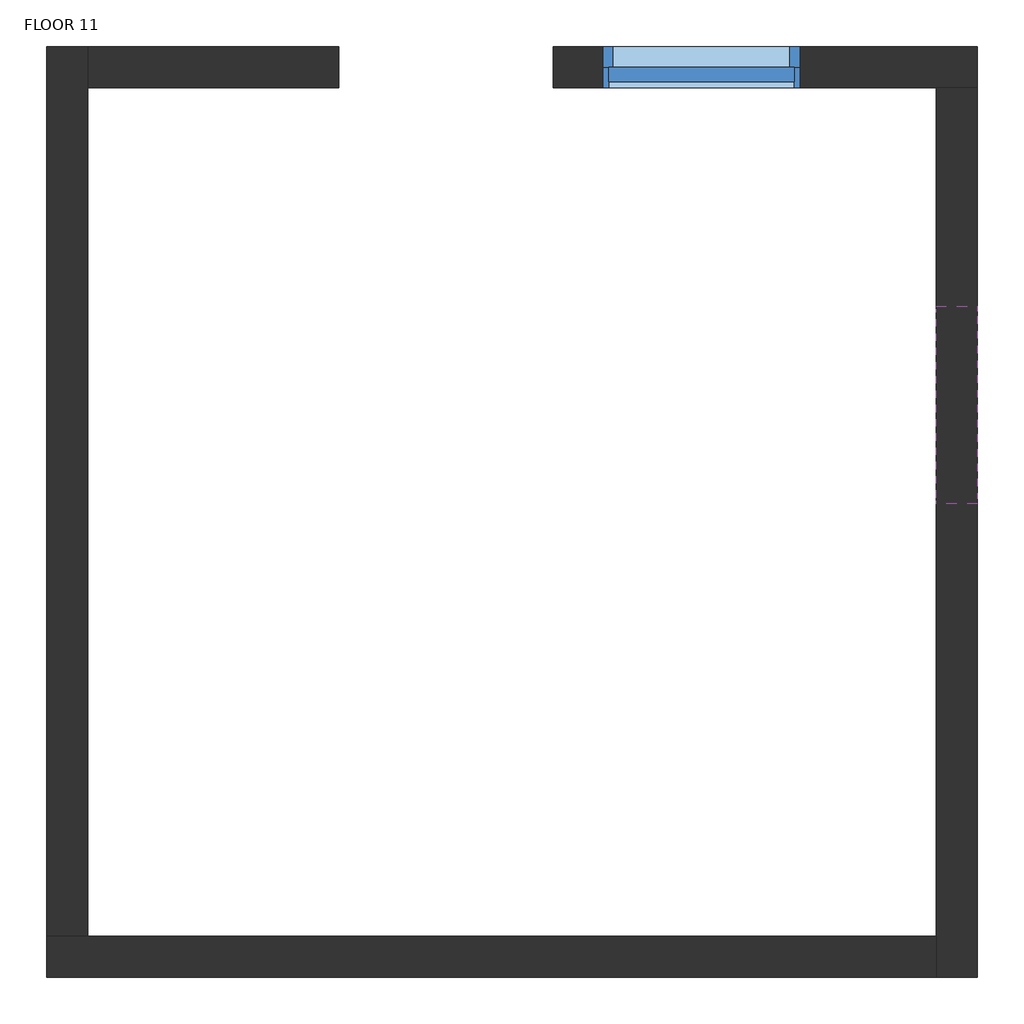
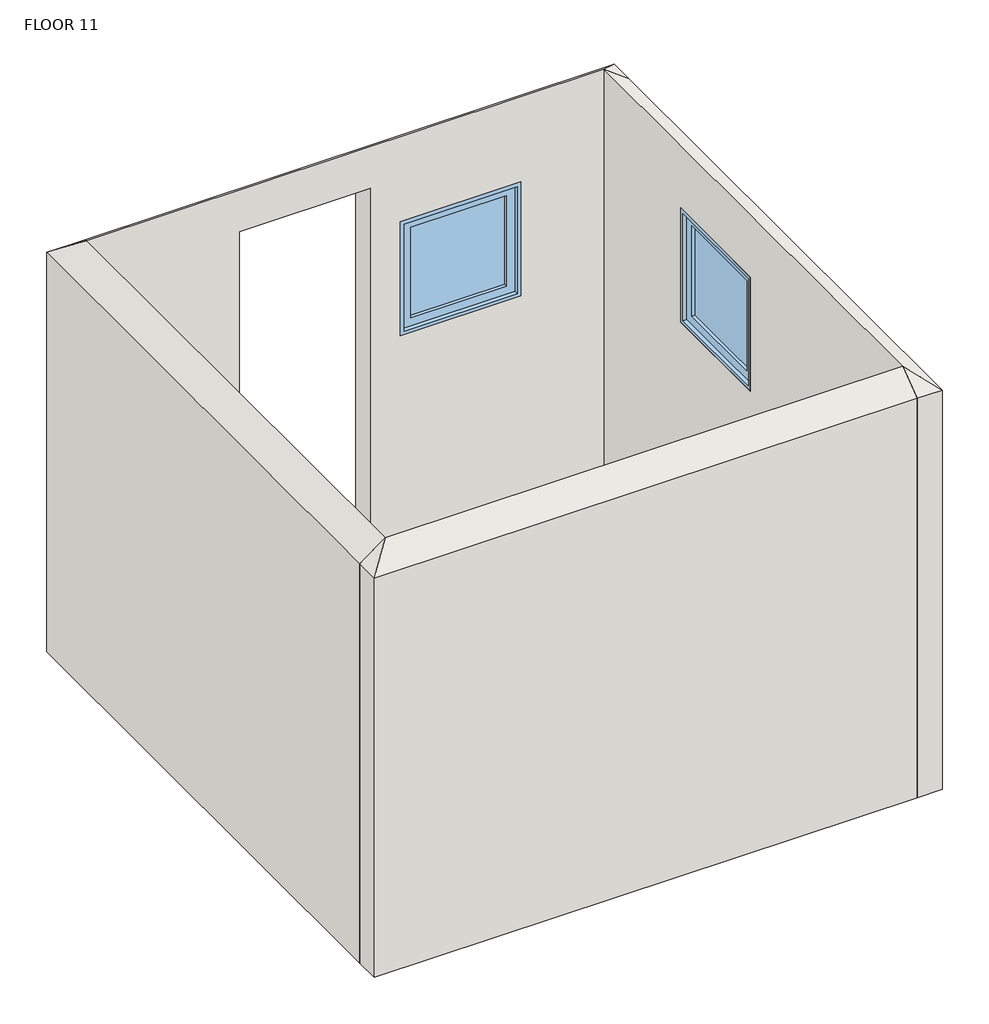
# One storey, incomplete: 4 walls, 2 windows.
"""IFC4 building model written with IfcOpenShell, lengths in millimetres."""

from ifc_helpers import new_model, si_unit, origin, place, context, project, spatial, faceted_brep, transform, mapped, element, save
from components import window_d757e824

model = new_model("IFC4")

# Units and contexts
model_context = context("Model", 3, world=origin())
ifc_project = project(units=[si_unit("LENGTHUNIT", "METRE", prefix="MILLI")], contexts=[model_context])

# Site, building, storey
site = spatial("IfcSite", under=ifc_project)
building = spatial("IfcBuilding", under=site)
storey = spatial("IfcBuildingStorey", under=building, Name="FLOOR 11", Elevation=15945.1725604)

# Walls
placement = place(None, origin())
element("IfcWall", 1, ObjectType="Inner Wall 5\"", at=placement, inside=storey, context=model_context, shape_type="Brep", body=[
    faceted_brep([(-6351.8094527, -6116.7242565, 15945.1725604), (-3608.6094527, -6116.7242565, 15945.1725604), (-3608.6094527, -6116.7242565, 18078.7725604), (-6351.8094527, -6116.7242565, 18078.7725604), (-6351.8094527, -5989.7242565, 15945.1725604), (-6351.8094527, -5989.7242565, 18078.7725604), (-6224.8094527, -5989.7242565, 18174.0225604), (-3608.6094527, -5989.7242565, 18174.0225604), (-3608.6094527, -5989.7242565, 15945.1725604), (-6224.8094527, -5989.7242565, 15945.1725604)], [[[0, 1, 2, 3]], [[4, 5, 6, 7, 8, 9]], [[1, 0, 4, 9, 8]], [[0, 3, 5, 4]], [[2, 1, 8, 7]], [[3, 2, 7, 6]], [[6, 5, 3]]]),
])
element("IfcWall", 2, ObjectType="Inner Wall 5\"", at=placement, inside=storey, context=model_context, shape_type="Brep", body=[
    faceted_brep([(-6351.8094527, -3246.5242565, 15945.1725604), (-6351.8094527, -5989.7242565, 15945.1725604), (-6351.8094527, -5989.7242565, 18078.7725604), (-6351.8094527, -3246.5242565, 18078.7725604), (-6224.8094527, -3246.5242565, 15945.1725604), (-6224.8094527, -3246.5242565, 18078.7725604), (-6224.8094527, -3373.5242565, 18174.0225604), (-6224.8094527, -5989.7242565, 18174.0225604), (-6224.8094527, -5989.7242565, 15945.1725604), (-6224.8094527, -3373.5242565, 15945.1725604)], [[[0, 1, 2, 3]], [[4, 5, 6, 7, 8, 9]], [[1, 0, 4, 9, 8]], [[0, 3, 5, 4]], [[2, 1, 8, 7]], [[3, 2, 7, 6]], [[6, 5, 3]]]),
])
element("IfcWall", 3, ObjectType="Inner Wall 5\"", at=placement, inside=storey, context=model_context, shape_type="Brep", body=[
    faceted_brep([(-3481.6094527, -3246.5242565, 18078.7725604), (-3481.6094527, -3246.5242565, 15945.1725604), (-4789.7094527, -3246.5242565, 15945.1725604), (-4789.7094527, -3246.5242565, 17951.7725604), (-5450.1094527, -3246.5242565, 17951.7725604), (-5450.1094527, -3246.5242565, 15945.1725604), (-6224.8094527, -3246.5242565, 15945.1725604), (-6224.8094527, -3246.5242565, 18078.7725604), (-4637.3094527, -3246.5242565, 17719.1457055), (-4637.3094527, -3246.5242565, 17109.5457055), (-4027.7094527, -3246.5242565, 17109.5457055), (-4027.7094527, -3246.5242565, 17719.1457055), (-3481.6094527, -3373.5242565, 15945.1725604), (-3481.6094527, -3373.5242565, 18078.7725604), (-3608.6094527, -3373.5242565, 18174.0225604), (-6224.8094527, -3373.5242565, 18174.0225604), (-6224.8094527, -3373.5242565, 15945.1725604), (-5450.1094527, -3373.5242565, 15945.1725604), (-5450.1094527, -3373.5242565, 17951.7725604), (-4789.7094527, -3373.5242565, 17951.7725604), (-4789.7094527, -3373.5242565, 15945.1725604), (-3608.6094527, -3373.5242565, 15945.1725604), (-4637.3094527, -3373.5242565, 17719.1457055), (-4027.7094527, -3373.5242565, 17719.1457055), (-4027.7094527, -3373.5242565, 17109.5457055), (-4637.3094527, -3373.5242565, 17109.5457055)], [[[0, 1, 2, 3, 4, 5, 6, 7], [8, 9, 10, 11]], [[12, 13, 14, 15, 16, 17, 18, 19, 20, 21], [22, 23, 24, 25]], [[1, 12, 21, 20, 2]], [[16, 6, 5, 17]], [[1, 0, 13, 12]], [[7, 6, 16, 15]], [[0, 7, 15, 14]], [[13, 0, 14]], [[19, 3, 2, 20]], [[3, 19, 18, 4]], [[4, 18, 17, 5]], [[9, 8, 22, 25]], [[10, 9, 25, 24]], [[11, 10, 24, 23]], [[8, 11, 23, 22]]]),
])
element("IfcWall", 4, ObjectType="Inner Wall 5\"", at=placement, inside=storey, context=model_context, shape_type="Brep", body=[
    faceted_brep([(-3481.6094527, -6116.7242565, 15945.1725604), (-3481.6094527, -3373.5242565, 15945.1725604), (-3481.6094527, -3373.5242565, 18078.7725604), (-3481.6094527, -6116.7242565, 18078.7725604), (-3481.6094527, -4046.6242565, 17840.991536), (-3481.6094527, -4046.6242565, 17231.391536), (-3481.6094527, -4656.2242565, 17231.391536), (-3481.6094527, -4656.2242565, 17840.991536), (-3608.6094527, -6116.7242565, 15945.1725604), (-3608.6094527, -6116.7242565, 18078.7725604), (-3608.6094527, -5989.7242565, 18174.0225604), (-3608.6094527, -3373.5242565, 18174.0225604), (-3608.6094527, -3373.5242565, 15945.1725604), (-3608.6094527, -5989.7242565, 15945.1725604), (-3608.6094527, -4046.6242565, 17840.991536), (-3608.6094527, -4656.2242565, 17840.991536), (-3608.6094527, -4656.2242565, 17231.391536), (-3608.6094527, -4046.6242565, 17231.391536)], [[[0, 1, 2, 3], [4, 5, 6, 7]], [[8, 9, 10, 11, 12, 13], [14, 15, 16, 17]], [[1, 0, 8, 13, 12]], [[0, 3, 9, 8]], [[2, 1, 12, 11]], [[3, 2, 11, 10]], [[10, 9, 3]], [[5, 4, 14, 17]], [[6, 5, 17, 16]], [[7, 6, 16, 15]], [[4, 7, 15, 14]]]),
])

# Windows
window_shape = window_d757e824(model_context)
element("IfcWindow", 5, ObjectType="Fixed : 24\" x 24\"", at=placement, inside=storey, context=model_context, shape_type="MappedRepresentation", body=[
    mapped(window_shape, transform((-3545.1094527, -4313.3242565, 16316.991536), x_axis=(0.0, 1.0, 0.0), y_axis=(-1.0, 0.0, 0.0), z_axis=(0.0, 0.0, 1.0))),
])
element("IfcWindow", 6, ObjectType="Fixed : 24\" x 24\"", at=placement, inside=storey, context=model_context, shape_type="MappedRepresentation", body=[
    mapped(window_shape, transform((-4370.6094527, -3310.0242565, 16195.1457055), x_axis=(-1.0, 0.0, 0.0), y_axis=(0.0, -1.0, 0.0), z_axis=(0.0, 0.0, 1.0))),
])

save(model, "model.ifc")

# Revit data of these elements
# Type "Inner Wall 5\""
#   Assembly Code = "B2010"
#   Layers, outside or top first: 0' - 5" "wall paint" (function 1)
# Type "Fixed : 24\" x 24\""
#   Type Mark = "3"
#   Construction Type Id = "GSP4R"
#   Assembly Code = "B2020100"
#   Analytic Construction = "1/8 in Pilkington single glazing"
#   Visual Light Transmittance = 0.9
#   Solar Heat Gain Coefficient = 0.78
#   Heat Transfer Coefficient (U) = 0.6496 BTU/(h·ft²·°F)
#   Height = 2' - 0"
#   Default Sill Height = 3' - 0"
#   Width = 2' - 0"
#   Window Inset = 0' - 0 3/4"
#   Define Thermal Properties by = 1
#   Define Thermal Properties by = 1
#   Glass Pane Material = Glass
#   Sash Material = Sash
#   Wall Closure = (empty or 0)
# Elements 1, 2, 3, 4 (IfcWall, "Inner Wall 5\"")
#   Top Offset = 0' - 0"
#   Base Offset = 0' - 0"
#   Unconnected Height = 7' - 0"
#   wall height = 7' - 0"
#   Phase Created = New Construction
#   Base Constraint = FLOOR 11
#   Materials on its faces: "wall paint", "Clad - White"
# Element 5 (IfcWindow, "Fixed : 24\" x 24\"")
#   Mark = "185"
#   Phase Created = New Construction
#   Materials on its faces: "Sash", "Glass"
# Element 6 (IfcWindow, "Fixed : 24\" x 24\"")
#   Mark = "186"
#   Phase Created = New Construction
#   Materials on its faces: "Sash", "Glass"
# Materials
#   "wall paint": class "Generic", colour RGB 120 120 120, transparency 0, Cost = 0
#   "Glass": class "Glass", colour RGB 0 128 192, transparency 0.75, Description = "Soda Lime Glass", Cost = 0
#   "Sash": class "Wood", colour RGB 224 178 126, transparency 0, Cost = 0
#   "Clad - White": class "Wood", colour RGB 242 242 238, transparency 0, Cost = 0
